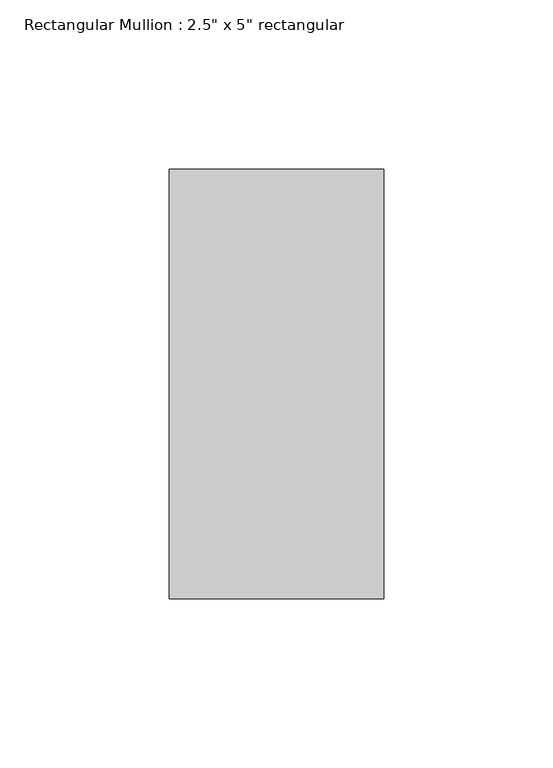
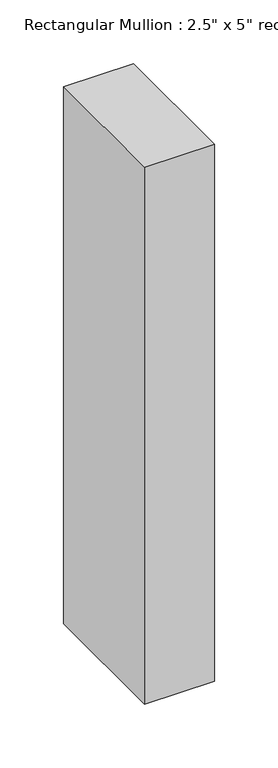
"""IFC4 building model written with IfcOpenShell, lengths in millimetres: member geometry."""

from ifc_helpers import new_model, si_unit, frame, origin, place, context, project, spatial, polyline, outline, extrude, source, transform, mapped, element, save


def member_0b7646a3(model_context):
    return source(origin(), model_context, "Body", "SweptSolid", [
        extrude(outline(polyline([(0.0, 63.5), (0.0, -63.5), (-63.5, -63.5), (-63.5, 63.5), (0.0, 63.5)])), frame((0.0, 0.0, -514.35), z_axis=(0.0, 0.0, 1.0), x_axis=(1.0, 0.0, 0.0)), (0.0, 0.0, 1.0), 514.35),
    ])


if __name__ == "__main__":
    model = new_model("IFC4")
    model_context = context("Model", 3, world=origin())
    ifc_project = project(units=[si_unit("LENGTHUNIT", "METRE", prefix="MILLI")], contexts=[model_context])
    site = spatial("IfcSite", under=ifc_project)
    building = spatial("IfcBuilding", under=site)
    placement = place(None, origin())
    member_shape = member_0b7646a3(model_context)
    element("IfcMember", 1, ObjectType="Rectangular Mullion : 2.5\" x 5\" rectangular", at=placement, inside=building, context=model_context, shape_type="MappedRepresentation", body=[
        mapped(member_shape, transform((0.0, 0.0, 0.0), x_axis=(1.0, 0.0, 0.0), y_axis=(0.0, 1.0, 0.0), z_axis=(0.0, 0.0, 1.0))),
    ])
    save(model, "model.ifc")

# Revit data of these elements
# Type "Rectangular Mullion : 2.5\" x 5\" rectangular"
#   built-in parameter 1007304 = 0.416667 (stored number, unit not read)
#   built-in parameter 1007301 = 0.104167 (stored number, unit not read)
#   built-in parameter 1007300 = 0.104167 (stored number, unit not read)
# Element 1 (IfcMember, "Rectangular Mullion : 2.5\" x 5\" rectangular")
#   Materials on its faces: "Door - Frame"
# Materials
#   "Door - Frame": colour RGB 118 70 51, transparency 0, Cost = 0
